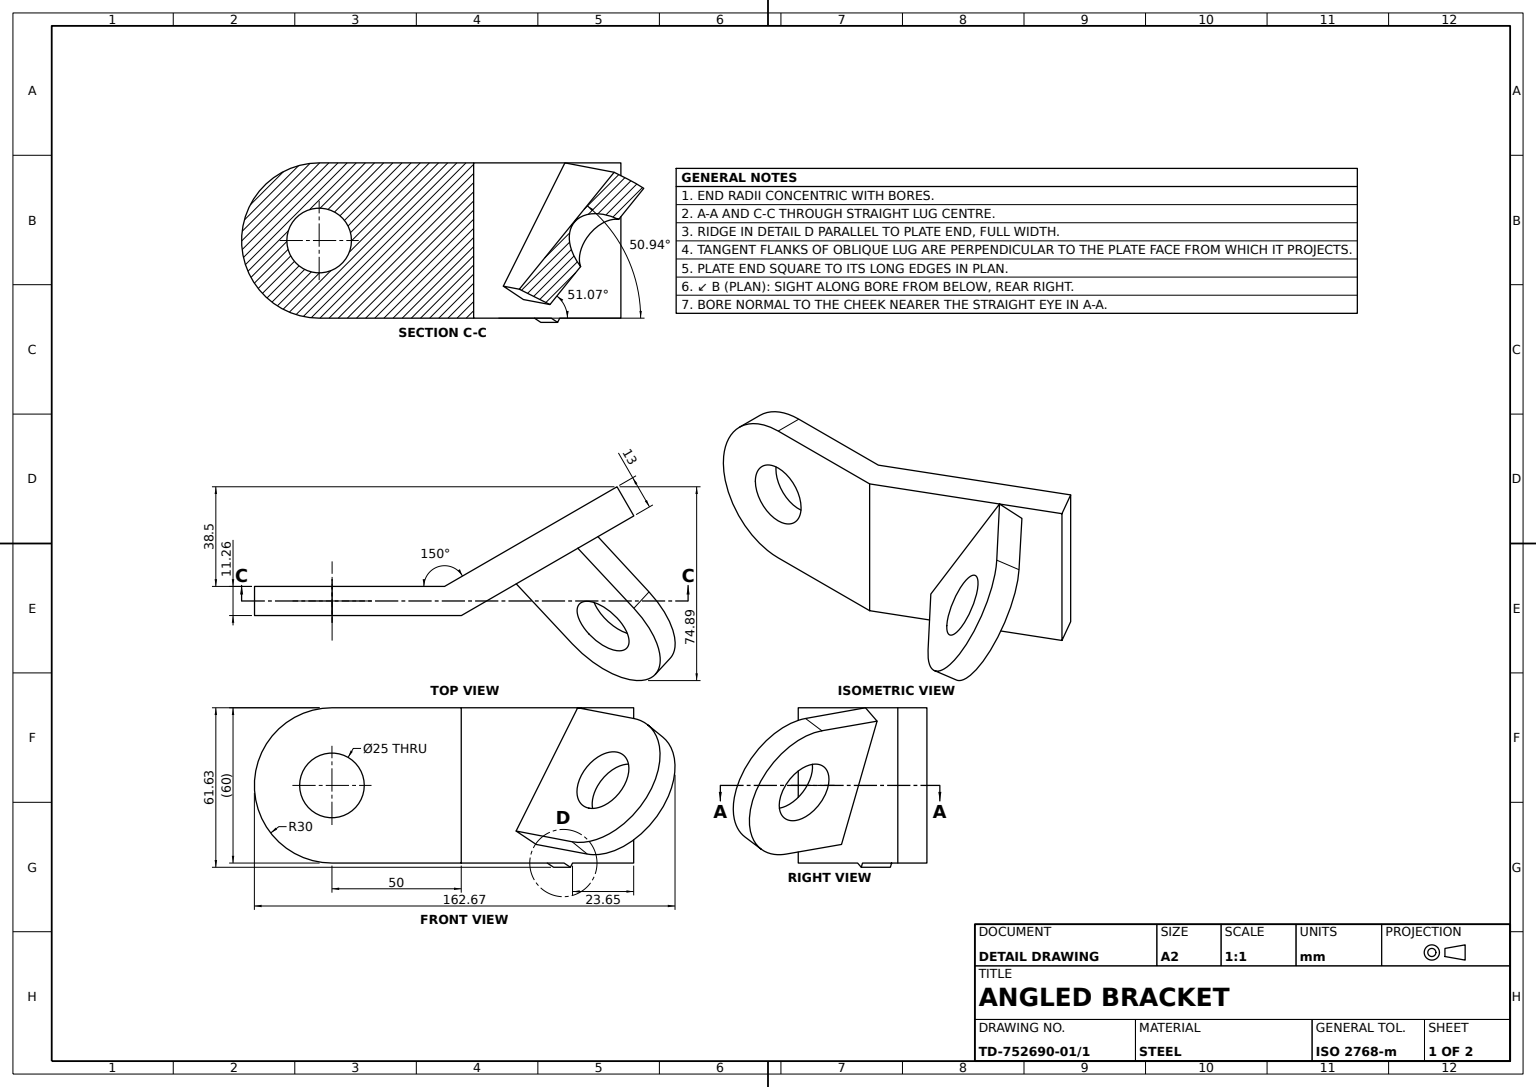
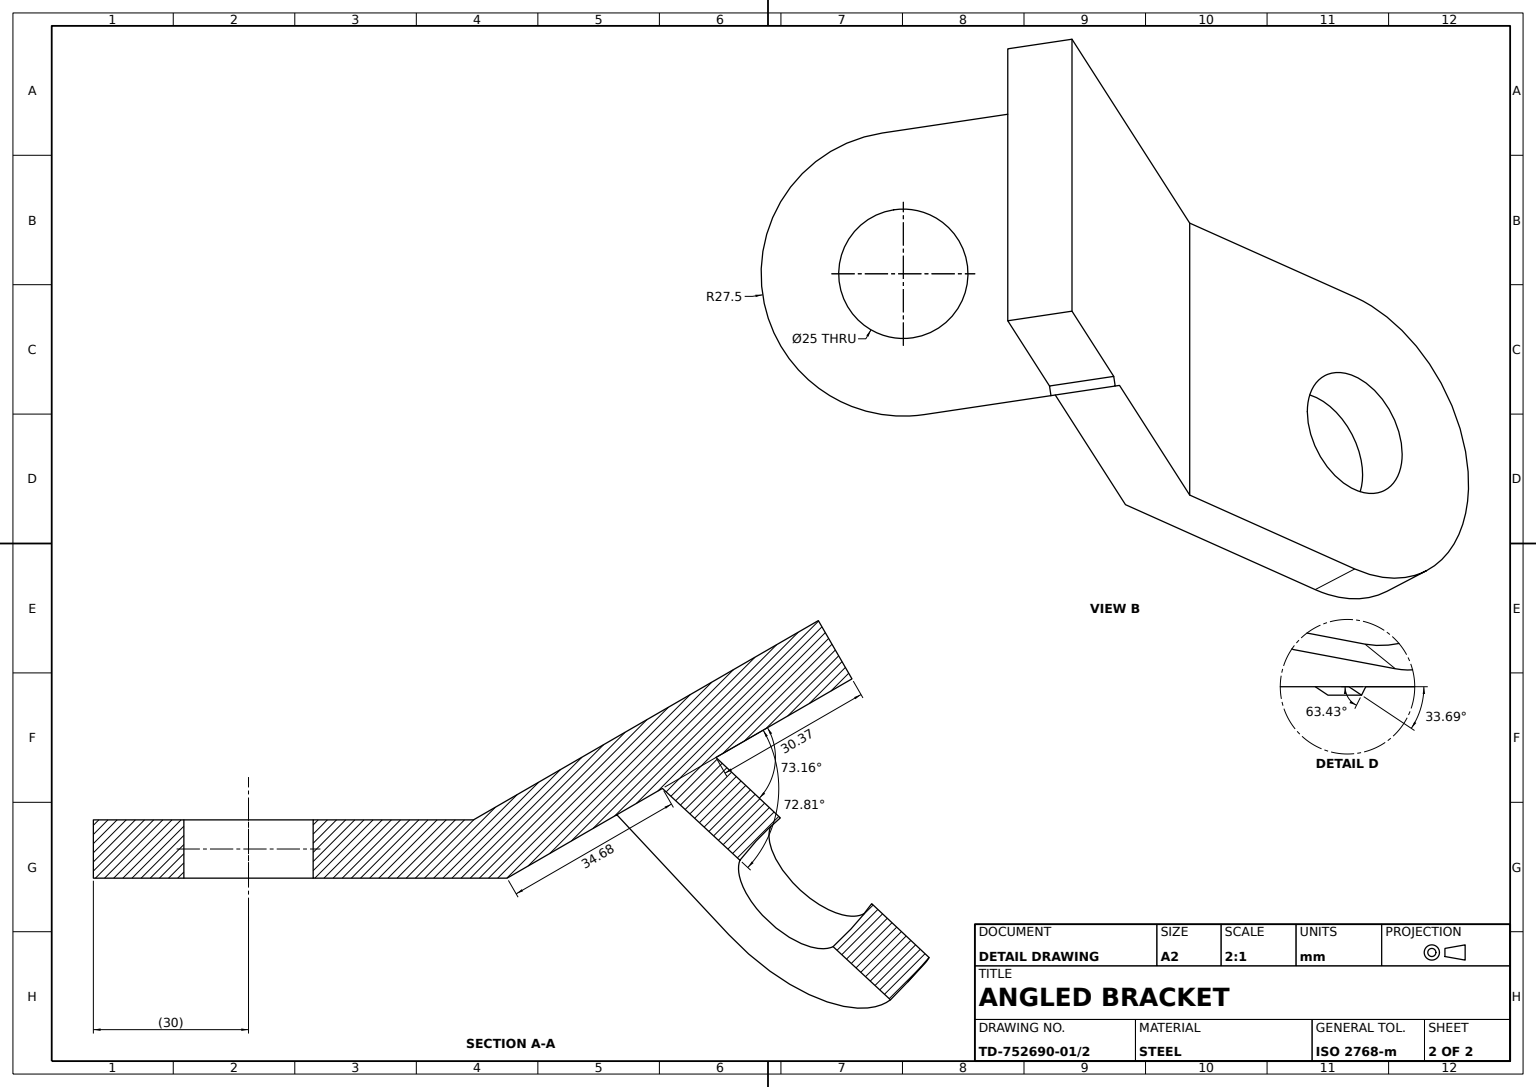
SolidWorks part; units mm, degrees
material "Plain Carbon Steel"
ref_plane "Front Plane" through (0, 0, 0) normal (0, 0, 1) x (1, 0, 0)
ref_plane "Top Plane" through (0, 0, 0) normal (0, 1, 0) x (1, 0, 0)
ref_plane "Right Plane" through (0, 0, 0) normal (1, 0, 0) x (0, 0, -1)
sketch "Base Plate Sketch" plane through (0, 0, 0) normal (0, 0, 1) x (1, 0, 0)
  line L1 (-38.5, 30) -> (38.5, 30)
  line L2 (-38.5, 30) -> (-38.5, -30)
  line L3 (-38.5, -30) -> (38.5, -30)
  line L4 (38.5, 30) -> (38.5, -30)
  line L5 (-38.5, 30) -> (38.5, -30) construction
  line L6 (-38.5, -30) -> (38.5, 30) construction
  point P0 (0, 0)
  dimension "D1" = 60
  dimension "D2" = 77
extrude "Base Plate 60x77x13" add sketch "Base Plate Sketch" along normal blind 13
sketch "Upper Lug Sketch" plane through (0, 0, 0) normal (0, 1, 0) x (1, 0, 0)
  line L8 (38.5, 0) -> (120.7724, -47.5)
  line L9 (120.7724, -47.5) -> (112.1122, -55.5)
  line L10 (112.1122, -55.5) -> (38.5, -13)
  line L12 (38.5, 0) -> (-38.5, 0)
  line L13 (-38.5, 0) -> (-38.5, -13)
  line L14 (-38.5, -13) -> (38.5, -13)
  line L15 (38.5, -13) -> (38.5, 0)
  line L16 (38.5, 0) -> (-38.5, 0)
  line L17 (-38.5, 0) -> (-38.5, -13)
  line L18 (-38.5, -13) -> (38.5, -13)
  line L19 (38.5, -13) -> (38.5, 0)
  dimension "D1" = 0
  dimension "D2" = 150
  dimension "D3" = 95
  dimension "D4" = 85
extrude "Upper Eye Lug" add sketch "Upper Lug Sketch" along normal mid plane 60 contours L19 L10 L9 L8
sketch "Upper Lug Cut Sketch" plane through (9.625, 0, -16.671) normal (0.5, 0, -0.866) x (-0.866, 0, -0.5)
  line L1 (-33.342, -30) -> (-128.342, -30) construction
  line L4 (-128.342, -30) -> (-33.342, -30)
  line L5 (-33.342, -30) -> (-33.342, 30)
  line L6 (-33.342, 30) -> (-128.342, 30)
  line L7 (-128.342, 30) -> (-128.342, -30)
  line L8 (-128.342, -30) -> (-33.342, -30)
  line L9 (-33.342, -30) -> (-33.342, 30)
  line L10 (-33.342, 30) -> (-128.342, 30)
  line L11 (-128.342, 30) -> (-128.342, -30)
  circle A0 centre (-83.342, 0) radius 30
  circle A1 centre (-83.342, 0) radius 12.5
  line M7 (-128.342, -30) -> (-33.342, -30)
  line M10 (-128.342, 30) -> (-128.342, -30)
  dimension "D2" = 60
  dimension "D3" = 25
  dimension "D4" = 50
  dimension "D5" = 30
  dimension "D1" = 0
extrude "Upper Lug Cut" cut sketch "Upper Lug Cut Sketch" against normal blind 13 contours A0 L10 M10 M7 | A1
sketch "Lower Lug Sketch" plane through (0, 0, 0) normal (0, 0, 1) x (1, 0, 0)
  line L0 (14, -17.6314) -> (-10.2487, -31.6314)
  line L1 (14, -17.6314) -> (-13.5, 30)
  line L2 (-10.2487, -31.6314) -> (-37.7487, 16)
  line L3 (-13.5, 30) -> (-37.7487, 16)
  line L4 (38.5, 30) -> (-38.5, 30) construction
  line L5 (-38.5, 30) -> (-38.5, -30) construction
  dimension "D1" = 60
  dimension "D2" = 25
  dimension "D3" = 28
  dimension "D4" = 55
extrude "Lower Eye Lug" add sketch "Lower Lug Sketch" against normal blind 62 and the other way blind 13
sketch "Lower Lug Profile Cut Sketch" plane through (-16.3654, 28.3457, 0) normal (-0.5, 0.866, 0) x (0.866, 0.5, 0)
  line L0 (-24.6913, 0) -> (-24.6913, 62) construction
  line L1 (3.3087, 0) -> (-18.342, 0) construction
  line L2 (-22.7683, 60) -> (-12.7683, 60)
  line L3 (-22.7683, 60) -> (-7.0441, 0)
  line L12 (-7.0441, 0) -> (3.3087, 0)
  line L13 (-12.7683, 60) -> (3.3087, 0)
  line L14 (-22.7683, 60) -> (3.3087, 0) construction
  line L15 (-7.0441, 0) -> (-12.7683, 60) construction
  line L16 (-24.6913, 0) -> (3.3087, 0) construction
  line L21 (-24.6913, 62) -> (-24.6913, 0)
  line L22 (-24.6913, 0) -> (3.3087, 0)
  line L23 (3.3087, 0) -> (3.3087, 62)
  line L24 (3.3087, 62) -> (-24.6913, 62)
  line L25 (-24.6913, 62) -> (-24.6913, 0)
  line L26 (-24.6913, 0) -> (3.3087, 0)
  line L27 (3.3087, 0) -> (3.3087, 62)
  line L28 (3.3087, 62) -> (-24.6913, 62)
  point P0 (-10.6834, 29.9395)
  line M13 (-24.6913, 62) -> (-24.6913, 0)
  line M14 (-24.6913, 0) -> (3.3087, 0)
  line M15 (3.3087, 0) -> (3.3087, 62)
  line M16 (3.3087, 62) -> (-24.6913, 62)
  dimension "D2" = 10
  dimension "D1" = 75
  dimension "D3" = 0
  dimension "D4" = 60
  dimension "D5" = 60
  dimension "D6" = 14.008
  dimension "D7" = 17.6472
  dimension "D8" = 32.0605
extrude "Lower Lug Profile Cut" cut sketch "Lower Lug Profile Cut Sketch" against normal blind 62 contours L2 L13 L3 M15 M16 M13 M14
sketch "Lower Lug Trim Sketch" plane through (2.6734, 1.5435, -0.8272) normal (0.8365, 0.483, -0.2588) x (-0.2241, -0.1294, -0.9659)
  line L0 (61.2602, 32.7308) -> (-0.8563, 32.7308) construction
  line L1 (-0.8563, 32.7308) -> (-0.8563, -22.2692) construction
  line L6 (61.2602, -22.2692) -> (61.2602, 32.7308)
  line L7 (61.2602, 32.7308) -> (-0.8563, 32.7308)
  line L8 (-0.8563, 32.7308) -> (-0.8563, -22.2692)
  line L9 (-0.8563, -22.2692) -> (61.2602, -22.2692)
  line L10 (61.2602, -22.2692) -> (61.2602, 32.7308)
  line L11 (61.2602, 32.7308) -> (-0.8563, 32.7308)
  line L12 (-0.8563, 32.7308) -> (-0.8563, -22.2692)
  line L13 (-0.8563, -22.2692) -> (61.2602, -22.2692)
  circle A0 centre (31.1437, 5.2308) radius 12.5
  circle A1 centre (31.1437, 5.2308) radius 27.5
  line M1 (61.2602, -22.2692) -> (61.2602, 32.7308)
  line M2 (61.2602, 32.7308) -> (-0.8563, 32.7308)
  dimension "D1" = 55
  dimension "D2" = 25
  dimension "D3" = 32
  dimension "D4" = 0
extrude "Lower Lug Trim Cut" cut sketch "Lower Lug Trim Sketch" against normal blind 62 contours A1 L13 M1 M2 | A0
